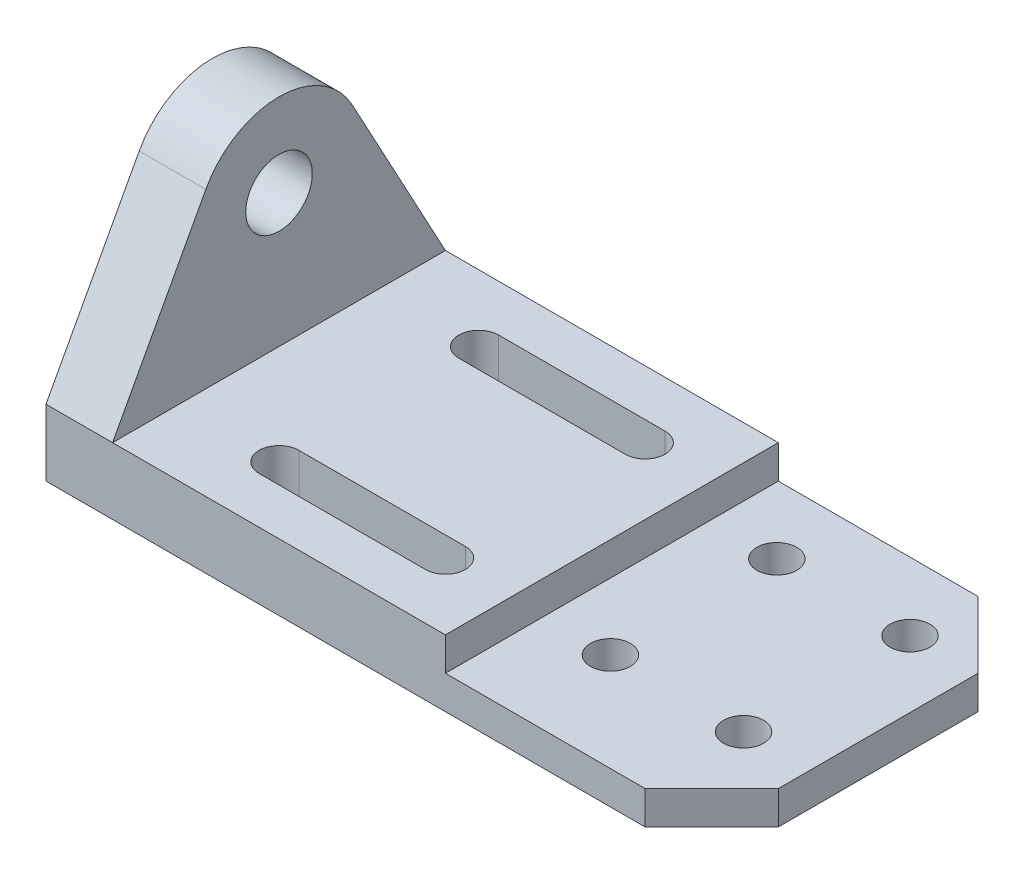
ISO-10303-21;
HEADER;
FILE_DESCRIPTION(('STEP AP214'),'2;1');
FILE_NAME('part.step','',(''),(''),'','','');
FILE_SCHEMA(('AUTOMOTIVE_DESIGN { 1 0 10303 214 1 1 1 1 }'));
ENDSEC;
DATA;
#1=APPLICATION_CONTEXT('core data for automotive mechanical design processes');
#2=APPLICATION_PROTOCOL_DEFINITION('international standard','automotive_design',2000,#1);
#3=PRODUCT_CONTEXT('',#1,'mechanical');
#4=PRODUCT('Part','Part','',(#3));
#5=PRODUCT_RELATED_PRODUCT_CATEGORY('part','',(#4));
#6=PRODUCT_DEFINITION_FORMATION('','',#4);
#7=PRODUCT_DEFINITION_CONTEXT('part definition',#1,'design');
#8=PRODUCT_DEFINITION('design','',#6,#7);
#9=PRODUCT_DEFINITION_SHAPE('','',#8);
#10=(LENGTH_UNIT() NAMED_UNIT(*) SI_UNIT(.MILLI.,.METRE.));
#11=(NAMED_UNIT(*) PLANE_ANGLE_UNIT() SI_UNIT($,.RADIAN.));
#12=(NAMED_UNIT(*) SI_UNIT($,.STERADIAN.) SOLID_ANGLE_UNIT());
#13=UNCERTAINTY_MEASURE_WITH_UNIT(LENGTH_MEASURE(1.E-05),#10,'distance_accuracy_value','');
#14=(GEOMETRIC_REPRESENTATION_CONTEXT(3) GLOBAL_UNCERTAINTY_ASSIGNED_CONTEXT((#13)) GLOBAL_UNIT_ASSIGNED_CONTEXT((#10,
#11,#12)) REPRESENTATION_CONTEXT('',''));
#15=CARTESIAN_POINT('',(0.,0.,0.));
#16=DIRECTION('',(0.,0.,1.));
#17=DIRECTION('',(1.,0.,0.));
#18=AXIS2_PLACEMENT_3D('',#15,#16,#17);
#19=CARTESIAN_POINT('',(0.,20.,0.));
#20=DIRECTION('',(0.,1.,0.));
#21=DIRECTION('',(0.,0.,1.));
#22=AXIS2_PLACEMENT_3D('',#19,#20,#21);
#23=PLANE('',#22);
#24=CARTESIAN_POINT('',(-50.,20.,30.));
#25=DIRECTION('',(0.,1.,0.));
#26=DIRECTION('',(0.,0.,1.));
#27=AXIS2_PLACEMENT_3D('',#24,#25,#26);
#28=CIRCLE('',#27,6.);
#29=CARTESIAN_POINT('',(-50.,20.,24.));
#30=VERTEX_POINT('',#29);
#31=CARTESIAN_POINT('',(-50.,20.,36.));
#32=VERTEX_POINT('',#31);
#33=EDGE_CURVE('E221',#30,#32,#28,.T.);
#34=ORIENTED_EDGE('',*,*,#33,.F.);
#35=DIRECTION('',(-1.,0.,0.));
#36=VECTOR('',#35,1.);
#37=CARTESIAN_POINT('',(-50.,20.,24.));
#38=LINE('',#37,#36);
#39=CARTESIAN_POINT('',(0.,20.,24.));
#40=VERTEX_POINT('',#39);
#41=EDGE_CURVE('E216',#40,#30,#38,.T.);
#42=ORIENTED_EDGE('',*,*,#41,.F.);
#43=CARTESIAN_POINT('',(0.,20.,30.));
#44=DIRECTION('',(0.,1.,0.));
#45=DIRECTION('',(0.,0.,1.));
#46=AXIS2_PLACEMENT_3D('',#43,#44,#45);
#47=CIRCLE('',#46,6.);
#48=CARTESIAN_POINT('',(0.,20.,36.));
#49=VERTEX_POINT('',#48);
#50=EDGE_CURVE('E227',#49,#40,#47,.T.);
#51=ORIENTED_EDGE('',*,*,#50,.F.);
#52=DIRECTION('',(1.,0.,0.));
#53=VECTOR('',#52,1.);
#54=CARTESIAN_POINT('',(-50.,20.,36.));
#55=LINE('',#54,#53);
#56=EDGE_CURVE('E228',#32,#49,#55,.T.);
#57=ORIENTED_EDGE('',*,*,#56,.F.);
#58=EDGE_LOOP('',(#34,#42,#51,#57));
#59=FACE_BOUND('',#58,.T.);
#60=CARTESIAN_POINT('',(-50.,20.,-30.));
#61=DIRECTION('',(0.,1.,0.));
#62=DIRECTION('',(0.,0.,-1.));
#63=AXIS2_PLACEMENT_3D('',#60,#61,#62);
#64=CIRCLE('',#63,6.);
#65=CARTESIAN_POINT('',(-50.,20.,-36.));
#66=VERTEX_POINT('',#65);
#67=CARTESIAN_POINT('',(-50.,20.,-24.));
#68=VERTEX_POINT('',#67);
#69=EDGE_CURVE('E209',#66,#68,#64,.T.);
#70=ORIENTED_EDGE('',*,*,#69,.F.);
#71=DIRECTION('',(-1.,0.,0.));
#72=VECTOR('',#71,1.);
#73=CARTESIAN_POINT('',(-50.,20.,-36.));
#74=LINE('',#73,#72);
#75=CARTESIAN_POINT('',(0.,20.,-36.));
#76=VERTEX_POINT('',#75);
#77=EDGE_CURVE('E250',#76,#66,#74,.T.);
#78=ORIENTED_EDGE('',*,*,#77,.F.);
#79=CARTESIAN_POINT('',(0.,20.,-30.));
#80=DIRECTION('',(0.,1.,0.));
#81=DIRECTION('',(0.,0.,-1.));
#82=AXIS2_PLACEMENT_3D('',#79,#80,#81);
#83=CIRCLE('',#82,6.);
#84=CARTESIAN_POINT('',(0.,20.,-24.));
#85=VERTEX_POINT('',#84);
#86=EDGE_CURVE('E265',#85,#76,#83,.T.);
#87=ORIENTED_EDGE('',*,*,#86,.F.);
#88=DIRECTION('',(1.,0.,0.));
#89=VECTOR('',#88,1.);
#90=CARTESIAN_POINT('',(-50.,20.,-24.));
#91=LINE('',#90,#89);
#92=EDGE_CURVE('E259',#68,#85,#91,.T.);
#93=ORIENTED_EDGE('',*,*,#92,.F.);
#94=EDGE_LOOP('',(#70,#78,#87,#93));
#95=FACE_BOUND('',#94,.T.);
#96=DIRECTION('',(-1.,0.,0.));
#97=VECTOR('',#96,1.);
#98=CARTESIAN_POINT('',(-100.,20.,-50.));
#99=LINE('',#98,#97);
#100=CARTESIAN_POINT('',(20.,20.,-50.));
#101=VERTEX_POINT('',#100);
#102=CARTESIAN_POINT('',(-80.,20.,-50.));
#103=VERTEX_POINT('',#102);
#104=EDGE_CURVE('E276',#101,#103,#99,.T.);
#105=ORIENTED_EDGE('',*,*,#104,.T.);
#106=DIRECTION('',(0.,0.,1.));
#107=VECTOR('',#106,1.);
#108=CARTESIAN_POINT('',(-80.,20.,-50.));
#109=LINE('',#108,#107);
#110=CARTESIAN_POINT('',(-80.,20.,50.));
#111=VERTEX_POINT('',#110);
#112=EDGE_CURVE('E192',#103,#111,#109,.T.);
#113=ORIENTED_EDGE('',*,*,#112,.T.);
#114=DIRECTION('',(1.,0.,0.));
#115=VECTOR('',#114,1.);
#116=CARTESIAN_POINT('',(-100.,20.,50.));
#117=LINE('',#116,#115);
#118=CARTESIAN_POINT('',(20.,20.,50.));
#119=VERTEX_POINT('',#118);
#120=EDGE_CURVE('E280',#111,#119,#117,.T.);
#121=ORIENTED_EDGE('',*,*,#120,.T.);
#122=DIRECTION('',(0.,0.,-1.));
#123=VECTOR('',#122,1.);
#124=CARTESIAN_POINT('',(20.,20.,-50.));
#125=LINE('',#124,#123);
#126=EDGE_CURVE('E277',#119,#101,#125,.T.);
#127=ORIENTED_EDGE('',*,*,#126,.T.);
#128=EDGE_LOOP('',(#105,#113,#121,#127));
#129=FACE_BOUND('',#128,.T.);
#130=ADVANCED_FACE('F41',(#59,#95,#129),#23,.T.);
#131=CARTESIAN_POINT('',(0.,10.,0.));
#132=DIRECTION('',(0.,-1.,0.));
#133=DIRECTION('',(0.,0.,-1.));
#134=AXIS2_PLACEMENT_3D('',#131,#132,#133);
#135=PLANE('',#134);
#136=CARTESIAN_POINT('',(40.,10.,20.4344291073049));
#137=DIRECTION('',(0.,1.,0.));
#138=DIRECTION('',(0.,0.,-1.));
#139=AXIS2_PLACEMENT_3D('',#136,#137,#138);
#140=CIRCLE('',#139,5.99999999999999);
#141=CARTESIAN_POINT('',(40.,10.,14.4344291073049));
#142=VERTEX_POINT('',#141);
#143=EDGE_CURVE('E355',#142,#142,#140,.T.);
#144=ORIENTED_EDGE('',*,*,#143,.F.);
#145=EDGE_LOOP('',(#144));
#146=FACE_BOUND('',#145,.T.);
#147=CARTESIAN_POINT('',(80.,10.,20.4344291073049));
#148=DIRECTION('',(0.,1.,0.));
#149=DIRECTION('',(0.,0.,-1.));
#150=AXIS2_PLACEMENT_3D('',#147,#148,#149);
#151=CIRCLE('',#150,5.99999999999998);
#152=CARTESIAN_POINT('',(80.,10.,14.4344291073049));
#153=VERTEX_POINT('',#152);
#154=EDGE_CURVE('E352',#153,#153,#151,.T.);
#155=ORIENTED_EDGE('',*,*,#154,.F.);
#156=EDGE_LOOP('',(#155));
#157=FACE_BOUND('',#156,.T.);
#158=CARTESIAN_POINT('',(80.,10.,-29.5655708926951));
#159=DIRECTION('',(0.,1.,0.));
#160=DIRECTION('',(0.,0.,1.));
#161=AXIS2_PLACEMENT_3D('',#158,#159,#160);
#162=CIRCLE('',#161,6.);
#163=CARTESIAN_POINT('',(80.,10.,-23.5655708926951));
#164=VERTEX_POINT('',#163);
#165=EDGE_CURVE('E353',#164,#164,#162,.T.);
#166=ORIENTED_EDGE('',*,*,#165,.F.);
#167=EDGE_LOOP('',(#166));
#168=FACE_BOUND('',#167,.T.);
#169=CARTESIAN_POINT('',(40.,10.,-29.5655708926951));
#170=DIRECTION('',(0.,1.,0.));
#171=DIRECTION('',(0.,0.,1.));
#172=AXIS2_PLACEMENT_3D('',#169,#170,#171);
#173=CIRCLE('',#172,6.);
#174=CARTESIAN_POINT('',(40.,10.,-23.5655708926951));
#175=VERTEX_POINT('',#174);
#176=EDGE_CURVE('E334',#175,#175,#173,.T.);
#177=ORIENTED_EDGE('',*,*,#176,.F.);
#178=EDGE_LOOP('',(#177));
#179=FACE_BOUND('',#178,.T.);
#180=DIRECTION('',(0.,0.,-1.));
#181=VECTOR('',#180,1.);
#182=CARTESIAN_POINT('',(100.,10.,50.));
#183=LINE('',#182,#181);
#184=CARTESIAN_POINT('',(100.,10.,30.));
#185=VERTEX_POINT('',#184);
#186=CARTESIAN_POINT('',(100.,10.,-29.9999999999999));
#187=VERTEX_POINT('',#186);
#188=EDGE_CURVE('E292',#185,#187,#183,.T.);
#189=ORIENTED_EDGE('',*,*,#188,.T.);
#190=DIRECTION('',(0.707106781186547,0.,0.707106781186549));
#191=VECTOR('',#190,1.);
#192=CARTESIAN_POINT('',(80.,10.,-50.));
#193=LINE('',#192,#191);
#194=CARTESIAN_POINT('',(80.,10.,-50.));
#195=VERTEX_POINT('',#194);
#196=EDGE_CURVE('E11',#187,#195,#193,.F.);
#197=ORIENTED_EDGE('',*,*,#196,.T.);
#198=DIRECTION('',(-1.,0.,0.));
#199=VECTOR('',#198,1.);
#200=CARTESIAN_POINT('',(-100.,10.,-50.));
#201=LINE('',#200,#199);
#202=CARTESIAN_POINT('',(20.,10.,-50.));
#203=VERTEX_POINT('',#202);
#204=EDGE_CURVE('E294',#195,#203,#201,.T.);
#205=ORIENTED_EDGE('',*,*,#204,.T.);
#206=DIRECTION('',(0.,0.,-1.));
#207=VECTOR('',#206,1.);
#208=CARTESIAN_POINT('',(20.,10.,-50.));
#209=LINE('',#208,#207);
#210=CARTESIAN_POINT('',(20.,10.,50.));
#211=VERTEX_POINT('',#210);
#212=EDGE_CURVE('E240',#211,#203,#209,.T.);
#213=ORIENTED_EDGE('',*,*,#212,.F.);
#214=DIRECTION('',(1.,0.,0.));
#215=VECTOR('',#214,1.);
#216=CARTESIAN_POINT('',(-100.,10.,50.));
#217=LINE('',#216,#215);
#218=CARTESIAN_POINT('',(79.9999999999999,10.,50.));
#219=VERTEX_POINT('',#218);
#220=EDGE_CURVE('E300',#211,#219,#217,.T.);
#221=ORIENTED_EDGE('',*,*,#220,.T.);
#222=DIRECTION('',(-0.707106781186549,0.,0.707106781186547));
#223=VECTOR('',#222,1.);
#224=CARTESIAN_POINT('',(100.,10.,30.));
#225=LINE('',#224,#223);
#226=EDGE_CURVE('E321',#219,#185,#225,.F.);
#227=ORIENTED_EDGE('',*,*,#226,.T.);
#228=EDGE_LOOP('',(#189,#197,#205,#213,#221,#227));
#229=FACE_BOUND('',#228,.T.);
#230=ADVANCED_FACE('F361',(#146,#157,#168,#179,#229),#135,.F.);
#231=CARTESIAN_POINT('',(100.,10.,50.));
#232=DIRECTION('',(-1.,0.,0.));
#233=DIRECTION('',(0.,0.,1.));
#234=AXIS2_PLACEMENT_3D('',#231,#232,#233);
#235=PLANE('',#234);
#236=DIRECTION('',(0.,0.,-1.));
#237=VECTOR('',#236,1.);
#238=CARTESIAN_POINT('',(100.,0.,50.));
#239=LINE('',#238,#237);
#240=CARTESIAN_POINT('',(100.,0.,30.));
#241=VERTEX_POINT('',#240);
#242=CARTESIAN_POINT('',(100.,0.,-29.9999999999999));
#243=VERTEX_POINT('',#242);
#244=EDGE_CURVE('E288',#241,#243,#239,.T.);
#245=ORIENTED_EDGE('',*,*,#244,.T.);
#246=DIRECTION('',(0.,1.,0.));
#247=VECTOR('',#246,1.);
#248=CARTESIAN_POINT('',(100.,10.,-29.9999999999999));
#249=LINE('',#248,#247);
#250=EDGE_CURVE('E51',#243,#187,#249,.T.);
#251=ORIENTED_EDGE('',*,*,#250,.T.);
#252=ORIENTED_EDGE('',*,*,#188,.F.);
#253=DIRECTION('',(0.,-1.,0.));
#254=VECTOR('',#253,1.);
#255=CARTESIAN_POINT('',(100.,10.,30.));
#256=LINE('',#255,#254);
#257=EDGE_CURVE('E314',#185,#241,#256,.T.);
#258=ORIENTED_EDGE('',*,*,#257,.T.);
#259=EDGE_LOOP('',(#245,#251,#252,#258));
#260=FACE_BOUND('',#259,.T.);
#261=ADVANCED_FACE('F368',(#260),#235,.F.);
#262=CARTESIAN_POINT('',(-100.,10.,-50.));
#263=DIRECTION('',(0.,0.,1.));
#264=DIRECTION('',(1.,0.,0.));
#265=AXIS2_PLACEMENT_3D('',#262,#263,#264);
#266=PLANE('',#265);
#267=ORIENTED_EDGE('',*,*,#204,.F.);
#268=DIRECTION('',(0.,-1.,0.));
#269=VECTOR('',#268,1.);
#270=CARTESIAN_POINT('',(80.,10.,-50.));
#271=LINE('',#270,#269);
#272=CARTESIAN_POINT('',(80.,0.,-50.));
#273=VERTEX_POINT('',#272);
#274=EDGE_CURVE('E323',#195,#273,#271,.T.);
#275=ORIENTED_EDGE('',*,*,#274,.T.);
#276=DIRECTION('',(-1.,0.,0.));
#277=VECTOR('',#276,1.);
#278=CARTESIAN_POINT('',(-100.,0.,-50.));
#279=LINE('',#278,#277);
#280=CARTESIAN_POINT('',(-100.,0.,-50.));
#281=VERTEX_POINT('',#280);
#282=EDGE_CURVE('E305',#273,#281,#279,.T.);
#283=ORIENTED_EDGE('',*,*,#282,.T.);
#284=DIRECTION('',(0.,-1.,0.));
#285=VECTOR('',#284,1.);
#286=CARTESIAN_POINT('',(-100.,10.,-50.));
#287=LINE('',#286,#285);
#288=CARTESIAN_POINT('',(-100.,20.,-50.));
#289=VERTEX_POINT('',#288);
#290=EDGE_CURVE('E313',#289,#281,#287,.T.);
#291=ORIENTED_EDGE('',*,*,#290,.F.);
#292=DIRECTION('',(-1.,0.,0.));
#293=VECTOR('',#292,1.);
#294=CARTESIAN_POINT('',(-80.,20.,-50.));
#295=LINE('',#294,#293);
#296=EDGE_CURVE('E188',#103,#289,#295,.T.);
#297=ORIENTED_EDGE('',*,*,#296,.F.);
#298=ORIENTED_EDGE('',*,*,#104,.F.);
#299=DIRECTION('',(0.,-1.,0.));
#300=VECTOR('',#299,1.);
#301=CARTESIAN_POINT('',(20.,20.,-50.));
#302=LINE('',#301,#300);
#303=EDGE_CURVE('E285',#101,#203,#302,.T.);
#304=ORIENTED_EDGE('',*,*,#303,.T.);
#305=EDGE_LOOP('',(#267,#275,#283,#291,#297,#298,#304));
#306=FACE_BOUND('',#305,.T.);
#307=ADVANCED_FACE('F385',(#306),#266,.F.);
#308=CARTESIAN_POINT('',(-100.,10.,50.));
#309=DIRECTION('',(1.,0.,0.));
#310=DIRECTION('',(0.,0.,-1.));
#311=AXIS2_PLACEMENT_3D('',#308,#309,#310);
#312=PLANE('',#311);
#313=DIRECTION('',(0.,0.,1.));
#314=VECTOR('',#313,1.);
#315=CARTESIAN_POINT('',(-100.,0.,50.));
#316=LINE('',#315,#314);
#317=CARTESIAN_POINT('',(-100.,0.,50.));
#318=VERTEX_POINT('',#317);
#319=EDGE_CURVE('E303',#281,#318,#316,.T.);
#320=ORIENTED_EDGE('',*,*,#319,.T.);
#321=DIRECTION('',(0.,-1.,0.));
#322=VECTOR('',#321,1.);
#323=CARTESIAN_POINT('',(-100.,10.,50.));
#324=LINE('',#323,#322);
#325=CARTESIAN_POINT('',(-100.,20.,50.));
#326=VERTEX_POINT('',#325);
#327=EDGE_CURVE('E297',#326,#318,#324,.T.);
#328=ORIENTED_EDGE('',*,*,#327,.F.);
#329=DIRECTION('',(0.,0.879991518173248,-0.474989397716561));
#330=VECTOR('',#329,1.);
#331=CARTESIAN_POINT('',(-100.,71.874734942914,21.9997879543312));
#332=LINE('',#331,#330);
#333=CARTESIAN_POINT('',(-100.,71.874734942914,21.9997879543312));
#334=VERTEX_POINT('',#333);
#335=EDGE_CURVE('E193',#326,#334,#332,.T.);
#336=ORIENTED_EDGE('',*,*,#335,.T.);
#337=CARTESIAN_POINT('',(-100.,60.,0.));
#338=DIRECTION('',(-1.,0.,0.));
#339=DIRECTION('',(0.,0.,1.));
#340=AXIS2_PLACEMENT_3D('',#337,#338,#339);
#341=CIRCLE('',#340,25.);
#342=CARTESIAN_POINT('',(-100.,71.874734942914,-21.9997879543312));
#343=VERTEX_POINT('',#342);
#344=EDGE_CURVE('E202',#334,#343,#341,.T.);
#345=ORIENTED_EDGE('',*,*,#344,.T.);
#346=DIRECTION('',(0.,-0.879991518173249,-0.47498939771656));
#347=VECTOR('',#346,1.);
#348=CARTESIAN_POINT('',(-100.,71.874734942914,-21.9997879543312));
#349=LINE('',#348,#347);
#350=EDGE_CURVE('E182',#343,#289,#349,.T.);
#351=ORIENTED_EDGE('',*,*,#350,.T.);
#352=ORIENTED_EDGE('',*,*,#290,.T.);
#353=EDGE_LOOP('',(#320,#328,#336,#345,#351,#352));
#354=FACE_BOUND('',#353,.T.);
#355=CARTESIAN_POINT('',(-100.,60.,0.));
#356=DIRECTION('',(-1.,0.,0.));
#357=DIRECTION('',(0.,0.,1.));
#358=AXIS2_PLACEMENT_3D('',#355,#356,#357);
#359=CIRCLE('',#358,10.);
#360=CARTESIAN_POINT('',(-100.,60.,10.));
#361=VERTEX_POINT('',#360);
#362=EDGE_CURVE('E199',#361,#361,#359,.T.);
#363=ORIENTED_EDGE('',*,*,#362,.F.);
#364=EDGE_LOOP('',(#363));
#365=FACE_BOUND('',#364,.T.);
#366=ADVANCED_FACE('F393',(#354,#365),#312,.F.);
#367=CARTESIAN_POINT('',(-100.,10.,50.));
#368=DIRECTION('',(0.,0.,-1.));
#369=DIRECTION('',(-1.,0.,0.));
#370=AXIS2_PLACEMENT_3D('',#367,#368,#369);
#371=PLANE('',#370);
#372=DIRECTION('',(1.,0.,0.));
#373=VECTOR('',#372,1.);
#374=CARTESIAN_POINT('',(-100.,0.,50.));
#375=LINE('',#374,#373);
#376=CARTESIAN_POINT('',(79.9999999999999,0.,50.));
#377=VERTEX_POINT('',#376);
#378=EDGE_CURVE('E293',#318,#377,#375,.T.);
#379=ORIENTED_EDGE('',*,*,#378,.T.);
#380=DIRECTION('',(0.,1.,0.));
#381=VECTOR('',#380,1.);
#382=CARTESIAN_POINT('',(79.9999999999999,10.,50.));
#383=LINE('',#382,#381);
#384=EDGE_CURVE('E317',#377,#219,#383,.T.);
#385=ORIENTED_EDGE('',*,*,#384,.T.);
#386=ORIENTED_EDGE('',*,*,#220,.F.);
#387=DIRECTION('',(0.,-1.,0.));
#388=VECTOR('',#387,1.);
#389=CARTESIAN_POINT('',(20.,20.,50.));
#390=LINE('',#389,#388);
#391=EDGE_CURVE('E289',#119,#211,#390,.T.);
#392=ORIENTED_EDGE('',*,*,#391,.F.);
#393=ORIENTED_EDGE('',*,*,#120,.F.);
#394=EDGE_CURVE('E273',#326,#111,#117,.T.);
#395=ORIENTED_EDGE('',*,*,#394,.F.);
#396=ORIENTED_EDGE('',*,*,#327,.T.);
#397=EDGE_LOOP('',(#379,#385,#386,#392,#393,#395,#396));
#398=FACE_BOUND('',#397,.T.);
#399=ADVANCED_FACE('F392',(#398),#371,.F.);
#400=CARTESIAN_POINT('',(0.,0.,0.));
#401=DIRECTION('',(0.,-1.,0.));
#402=DIRECTION('',(0.,0.,-1.));
#403=AXIS2_PLACEMENT_3D('',#400,#401,#402);
#404=PLANE('',#403);
#405=CARTESIAN_POINT('',(40.,0.,20.4344291073049));
#406=DIRECTION('',(0.,-1.,0.));
#407=DIRECTION('',(0.,0.,-1.));
#408=AXIS2_PLACEMENT_3D('',#405,#406,#407);
#409=CIRCLE('',#408,5.99999999999999);
#410=CARTESIAN_POINT('',(40.,0.,14.4344291073049));
#411=VERTEX_POINT('',#410);
#412=EDGE_CURVE('E46',#411,#411,#409,.T.);
#413=ORIENTED_EDGE('',*,*,#412,.F.);
#414=EDGE_LOOP('',(#413));
#415=FACE_BOUND('',#414,.T.);
#416=CARTESIAN_POINT('',(80.,0.,20.4344291073049));
#417=DIRECTION('',(0.,-1.,0.));
#418=DIRECTION('',(0.,0.,-1.));
#419=AXIS2_PLACEMENT_3D('',#416,#417,#418);
#420=CIRCLE('',#419,5.99999999999998);
#421=CARTESIAN_POINT('',(80.,0.,14.4344291073049));
#422=VERTEX_POINT('',#421);
#423=EDGE_CURVE('E333',#422,#422,#420,.T.);
#424=ORIENTED_EDGE('',*,*,#423,.F.);
#425=EDGE_LOOP('',(#424));
#426=FACE_BOUND('',#425,.T.);
#427=CARTESIAN_POINT('',(80.,0.,-29.5655708926951));
#428=DIRECTION('',(0.,-1.,0.));
#429=DIRECTION('',(0.,0.,-1.));
#430=AXIS2_PLACEMENT_3D('',#427,#428,#429);
#431=CIRCLE('',#430,6.);
#432=CARTESIAN_POINT('',(80.,0.,-35.5655708926951));
#433=VERTEX_POINT('',#432);
#434=EDGE_CURVE('E335',#433,#433,#431,.T.);
#435=ORIENTED_EDGE('',*,*,#434,.F.);
#436=EDGE_LOOP('',(#435));
#437=FACE_BOUND('',#436,.T.);
#438=CARTESIAN_POINT('',(40.,0.,-29.5655708926951));
#439=DIRECTION('',(0.,-1.,0.));
#440=DIRECTION('',(0.,0.,-1.));
#441=AXIS2_PLACEMENT_3D('',#438,#439,#440);
#442=CIRCLE('',#441,6.);
#443=CARTESIAN_POINT('',(40.,0.,-35.5655708926951));
#444=VERTEX_POINT('',#443);
#445=EDGE_CURVE('E328',#444,#444,#442,.T.);
#446=ORIENTED_EDGE('',*,*,#445,.F.);
#447=EDGE_LOOP('',(#446));
#448=FACE_BOUND('',#447,.T.);
#449=CARTESIAN_POINT('',(-50.,0.,30.));
#450=DIRECTION('',(0.,1.,0.));
#451=DIRECTION('',(0.,0.,1.));
#452=AXIS2_PLACEMENT_3D('',#449,#450,#451);
#453=CIRCLE('',#452,6.);
#454=CARTESIAN_POINT('',(-50.,0.,24.));
#455=VERTEX_POINT('',#454);
#456=CARTESIAN_POINT('',(-50.,0.,36.));
#457=VERTEX_POINT('',#456);
#458=EDGE_CURVE('E215',#455,#457,#453,.T.);
#459=ORIENTED_EDGE('',*,*,#458,.T.);
#460=DIRECTION('',(1.,0.,0.));
#461=VECTOR('',#460,1.);
#462=CARTESIAN_POINT('',(-50.,0.,36.));
#463=LINE('',#462,#461);
#464=CARTESIAN_POINT('',(0.,0.,36.));
#465=VERTEX_POINT('',#464);
#466=EDGE_CURVE('E214',#457,#465,#463,.T.);
#467=ORIENTED_EDGE('',*,*,#466,.T.);
#468=CARTESIAN_POINT('',(0.,0.,30.));
#469=DIRECTION('',(0.,1.,0.));
#470=DIRECTION('',(0.,0.,1.));
#471=AXIS2_PLACEMENT_3D('',#468,#469,#470);
#472=CIRCLE('',#471,6.);
#473=CARTESIAN_POINT('',(0.,0.,24.));
#474=VERTEX_POINT('',#473);
#475=EDGE_CURVE('E69',#465,#474,#472,.T.);
#476=ORIENTED_EDGE('',*,*,#475,.T.);
#477=DIRECTION('',(-1.,0.,0.));
#478=VECTOR('',#477,1.);
#479=CARTESIAN_POINT('',(-50.,0.,24.));
#480=LINE('',#479,#478);
#481=EDGE_CURVE('E219',#474,#455,#480,.T.);
#482=ORIENTED_EDGE('',*,*,#481,.T.);
#483=EDGE_LOOP('',(#459,#467,#476,#482));
#484=FACE_BOUND('',#483,.T.);
#485=CARTESIAN_POINT('',(-50.,0.,-30.));
#486=DIRECTION('',(0.,1.,0.));
#487=DIRECTION('',(0.,0.,-1.));
#488=AXIS2_PLACEMENT_3D('',#485,#486,#487);
#489=CIRCLE('',#488,6.);
#490=CARTESIAN_POINT('',(-50.,0.,-36.));
#491=VERTEX_POINT('',#490);
#492=CARTESIAN_POINT('',(-50.,0.,-24.));
#493=VERTEX_POINT('',#492);
#494=EDGE_CURVE('E244',#491,#493,#489,.T.);
#495=ORIENTED_EDGE('',*,*,#494,.T.);
#496=DIRECTION('',(1.,0.,0.));
#497=VECTOR('',#496,1.);
#498=CARTESIAN_POINT('',(-50.,0.,-24.));
#499=LINE('',#498,#497);
#500=CARTESIAN_POINT('',(0.,0.,-24.));
#501=VERTEX_POINT('',#500);
#502=EDGE_CURVE('E249',#493,#501,#499,.T.);
#503=ORIENTED_EDGE('',*,*,#502,.T.);
#504=CARTESIAN_POINT('',(0.,0.,-30.));
#505=DIRECTION('',(0.,1.,0.));
#506=DIRECTION('',(0.,0.,-1.));
#507=AXIS2_PLACEMENT_3D('',#504,#505,#506);
#508=CIRCLE('',#507,6.);
#509=CARTESIAN_POINT('',(0.,0.,-36.));
#510=VERTEX_POINT('',#509);
#511=EDGE_CURVE('E253',#501,#510,#508,.T.);
#512=ORIENTED_EDGE('',*,*,#511,.T.);
#513=DIRECTION('',(-1.,0.,0.));
#514=VECTOR('',#513,1.);
#515=CARTESIAN_POINT('',(-50.,0.,-36.));
#516=LINE('',#515,#514);
#517=EDGE_CURVE('E255',#510,#491,#516,.T.);
#518=ORIENTED_EDGE('',*,*,#517,.T.);
#519=EDGE_LOOP('',(#495,#503,#512,#518));
#520=FACE_BOUND('',#519,.T.);
#521=ORIENTED_EDGE('',*,*,#282,.F.);
#522=DIRECTION('',(-0.707106781186547,0.,-0.707106781186549));
#523=VECTOR('',#522,1.);
#524=CARTESIAN_POINT('',(65.0000000000001,0.,-64.9999999999999));
#525=LINE('',#524,#523);
#526=EDGE_CURVE('E326',#273,#243,#525,.F.);
#527=ORIENTED_EDGE('',*,*,#526,.T.);
#528=ORIENTED_EDGE('',*,*,#244,.F.);
#529=DIRECTION('',(0.707106781186549,0.,-0.707106781186547));
#530=VECTOR('',#529,1.);
#531=CARTESIAN_POINT('',(64.9999999999999,0.,65.0000000000001));
#532=LINE('',#531,#530);
#533=EDGE_CURVE('E320',#241,#377,#532,.F.);
#534=ORIENTED_EDGE('',*,*,#533,.T.);
#535=ORIENTED_EDGE('',*,*,#378,.F.);
#536=ORIENTED_EDGE('',*,*,#319,.F.);
#537=EDGE_LOOP('',(#521,#527,#528,#534,#535,#536));
#538=FACE_BOUND('',#537,.T.);
#539=ADVANCED_FACE('F387',(#415,#426,#437,#448,#484,#520,#538),#404,.T.);
#540=CARTESIAN_POINT('',(20.,20.,-50.));
#541=DIRECTION('',(-1.,0.,0.));
#542=DIRECTION('',(0.,0.,1.));
#543=AXIS2_PLACEMENT_3D('',#540,#541,#542);
#544=PLANE('',#543);
#545=ORIENTED_EDGE('',*,*,#212,.T.);
#546=ORIENTED_EDGE('',*,*,#303,.F.);
#547=ORIENTED_EDGE('',*,*,#126,.F.);
#548=ORIENTED_EDGE('',*,*,#391,.T.);
#549=EDGE_LOOP('',(#545,#546,#547,#548));
#550=FACE_BOUND('',#549,.T.);
#551=ADVANCED_FACE('F408',(#550),#544,.F.);
#552=CARTESIAN_POINT('',(100.,10.,30.));
#553=DIRECTION('',(-0.707106781186547,0.,-0.707106781186549));
#554=DIRECTION('',(0.,-1.,0.));
#555=AXIS2_PLACEMENT_3D('',#552,#553,#554);
#556=PLANE('',#555);
#557=ORIENTED_EDGE('',*,*,#226,.F.);
#558=ORIENTED_EDGE('',*,*,#384,.F.);
#559=ORIENTED_EDGE('',*,*,#533,.F.);
#560=ORIENTED_EDGE('',*,*,#257,.F.);
#561=EDGE_LOOP('',(#557,#558,#559,#560));
#562=FACE_BOUND('',#561,.T.);
#563=ADVANCED_FACE('F409',(#562),#556,.F.);
#564=CARTESIAN_POINT('',(80.,10.,-50.));
#565=DIRECTION('',(-0.707106781186549,0.,0.707106781186547));
#566=DIRECTION('',(0.,-1.,0.));
#567=AXIS2_PLACEMENT_3D('',#564,#565,#566);
#568=PLANE('',#567);
#569=ORIENTED_EDGE('',*,*,#196,.F.);
#570=ORIENTED_EDGE('',*,*,#250,.F.);
#571=ORIENTED_EDGE('',*,*,#526,.F.);
#572=ORIENTED_EDGE('',*,*,#274,.F.);
#573=EDGE_LOOP('',(#569,#570,#571,#572));
#574=FACE_BOUND('',#573,.T.);
#575=ADVANCED_FACE('F42',(#574),#568,.F.);
#576=CARTESIAN_POINT('',(-50.,0.,-30.));
#577=DIRECTION('',(0.,1.,0.));
#578=DIRECTION('',(0.,0.,1.));
#579=AXIS2_PLACEMENT_3D('',#576,#577,#578);
#580=CYLINDRICAL_SURFACE('',#579,6.);
#581=ORIENTED_EDGE('',*,*,#69,.T.);
#582=DIRECTION('',(0.,1.,0.));
#583=VECTOR('',#582,1.);
#584=CARTESIAN_POINT('',(-50.,0.,-24.));
#585=LINE('',#584,#583);
#586=EDGE_CURVE('E260',#493,#68,#585,.T.);
#587=ORIENTED_EDGE('',*,*,#586,.F.);
#588=ORIENTED_EDGE('',*,*,#494,.F.);
#589=DIRECTION('',(0.,1.,0.));
#590=VECTOR('',#589,1.);
#591=CARTESIAN_POINT('',(-50.,0.,-36.));
#592=LINE('',#591,#590);
#593=EDGE_CURVE('E230',#491,#66,#592,.T.);
#594=ORIENTED_EDGE('',*,*,#593,.T.);
#595=EDGE_LOOP('',(#581,#587,#588,#594));
#596=FACE_BOUND('',#595,.T.);
#597=ADVANCED_FACE('F428',(#596),#580,.F.);
#598=CARTESIAN_POINT('',(-50.,0.,-36.));
#599=DIRECTION('',(0.,0.,-1.));
#600=DIRECTION('',(-1.,0.,0.));
#601=AXIS2_PLACEMENT_3D('',#598,#599,#600);
#602=PLANE('',#601);
#603=ORIENTED_EDGE('',*,*,#77,.T.);
#604=ORIENTED_EDGE('',*,*,#593,.F.);
#605=ORIENTED_EDGE('',*,*,#517,.F.);
#606=DIRECTION('',(0.,1.,0.));
#607=VECTOR('',#606,1.);
#608=CARTESIAN_POINT('',(0.,0.,-36.));
#609=LINE('',#608,#607);
#610=EDGE_CURVE('E268',#510,#76,#609,.T.);
#611=ORIENTED_EDGE('',*,*,#610,.T.);
#612=EDGE_LOOP('',(#603,#604,#605,#611));
#613=FACE_BOUND('',#612,.T.);
#614=ADVANCED_FACE('F595',(#613),#602,.F.);
#615=CARTESIAN_POINT('',(0.,0.,-30.));
#616=DIRECTION('',(0.,1.,0.));
#617=DIRECTION('',(0.,0.,1.));
#618=AXIS2_PLACEMENT_3D('',#615,#616,#617);
#619=CYLINDRICAL_SURFACE('',#618,6.);
#620=ORIENTED_EDGE('',*,*,#86,.T.);
#621=ORIENTED_EDGE('',*,*,#610,.F.);
#622=ORIENTED_EDGE('',*,*,#511,.F.);
#623=DIRECTION('',(0.,1.,0.));
#624=VECTOR('',#623,1.);
#625=CARTESIAN_POINT('',(0.,0.,-24.));
#626=LINE('',#625,#624);
#627=EDGE_CURVE('E269',#501,#85,#626,.T.);
#628=ORIENTED_EDGE('',*,*,#627,.T.);
#629=EDGE_LOOP('',(#620,#621,#622,#628));
#630=FACE_BOUND('',#629,.T.);
#631=ADVANCED_FACE('F585',(#630),#619,.F.);
#632=CARTESIAN_POINT('',(-50.,0.,-24.));
#633=DIRECTION('',(0.,0.,1.));
#634=DIRECTION('',(1.,0.,0.));
#635=AXIS2_PLACEMENT_3D('',#632,#633,#634);
#636=PLANE('',#635);
#637=ORIENTED_EDGE('',*,*,#92,.T.);
#638=ORIENTED_EDGE('',*,*,#627,.F.);
#639=ORIENTED_EDGE('',*,*,#502,.F.);
#640=ORIENTED_EDGE('',*,*,#586,.T.);
#641=EDGE_LOOP('',(#637,#638,#639,#640));
#642=FACE_BOUND('',#641,.T.);
#643=ADVANCED_FACE('F572',(#642),#636,.F.);
#644=CARTESIAN_POINT('',(-50.,0.,30.));
#645=DIRECTION('',(0.,1.,0.));
#646=DIRECTION('',(0.,0.,1.));
#647=AXIS2_PLACEMENT_3D('',#644,#645,#646);
#648=CYLINDRICAL_SURFACE('',#647,6.);
#649=ORIENTED_EDGE('',*,*,#33,.T.);
#650=DIRECTION('',(0.,1.,0.));
#651=VECTOR('',#650,1.);
#652=CARTESIAN_POINT('',(-50.,0.,36.));
#653=LINE('',#652,#651);
#654=EDGE_CURVE('E224',#457,#32,#653,.T.);
#655=ORIENTED_EDGE('',*,*,#654,.F.);
#656=ORIENTED_EDGE('',*,*,#458,.F.);
#657=DIRECTION('',(0.,1.,0.));
#658=VECTOR('',#657,1.);
#659=CARTESIAN_POINT('',(-50.,0.,24.));
#660=LINE('',#659,#658);
#661=EDGE_CURVE('E233',#455,#30,#660,.T.);
#662=ORIENTED_EDGE('',*,*,#661,.T.);
#663=EDGE_LOOP('',(#649,#655,#656,#662));
#664=FACE_BOUND('',#663,.T.);
#665=ADVANCED_FACE('F567',(#664),#648,.F.);
#666=CARTESIAN_POINT('',(-50.,0.,24.));
#667=DIRECTION('',(0.,0.,-1.));
#668=DIRECTION('',(-1.,0.,0.));
#669=AXIS2_PLACEMENT_3D('',#666,#667,#668);
#670=PLANE('',#669);
#671=ORIENTED_EDGE('',*,*,#41,.T.);
#672=ORIENTED_EDGE('',*,*,#661,.F.);
#673=ORIENTED_EDGE('',*,*,#481,.F.);
#674=DIRECTION('',(0.,1.,0.));
#675=VECTOR('',#674,1.);
#676=CARTESIAN_POINT('',(0.,0.,24.));
#677=LINE('',#676,#675);
#678=EDGE_CURVE('E236',#474,#40,#677,.T.);
#679=ORIENTED_EDGE('',*,*,#678,.T.);
#680=EDGE_LOOP('',(#671,#672,#673,#679));
#681=FACE_BOUND('',#680,.T.);
#682=ADVANCED_FACE('F556',(#681),#670,.F.);
#683=CARTESIAN_POINT('',(0.,0.,30.));
#684=DIRECTION('',(0.,1.,0.));
#685=DIRECTION('',(0.,0.,1.));
#686=AXIS2_PLACEMENT_3D('',#683,#684,#685);
#687=CYLINDRICAL_SURFACE('',#686,6.);
#688=ORIENTED_EDGE('',*,*,#50,.T.);
#689=ORIENTED_EDGE('',*,*,#678,.F.);
#690=ORIENTED_EDGE('',*,*,#475,.F.);
#691=DIRECTION('',(0.,1.,0.));
#692=VECTOR('',#691,1.);
#693=CARTESIAN_POINT('',(0.,0.,36.));
#694=LINE('',#693,#692);
#695=EDGE_CURVE('E238',#465,#49,#694,.T.);
#696=ORIENTED_EDGE('',*,*,#695,.T.);
#697=EDGE_LOOP('',(#688,#689,#690,#696));
#698=FACE_BOUND('',#697,.T.);
#699=ADVANCED_FACE('F548',(#698),#687,.F.);
#700=CARTESIAN_POINT('',(-50.,0.,36.));
#701=DIRECTION('',(0.,0.,1.));
#702=DIRECTION('',(1.,0.,0.));
#703=AXIS2_PLACEMENT_3D('',#700,#701,#702);
#704=PLANE('',#703);
#705=ORIENTED_EDGE('',*,*,#56,.T.);
#706=ORIENTED_EDGE('',*,*,#695,.F.);
#707=ORIENTED_EDGE('',*,*,#466,.F.);
#708=ORIENTED_EDGE('',*,*,#654,.T.);
#709=EDGE_LOOP('',(#705,#706,#707,#708));
#710=FACE_BOUND('',#709,.T.);
#711=ADVANCED_FACE('F457',(#710),#704,.F.);
#712=CARTESIAN_POINT('',(-80.,60.,0.));
#713=DIRECTION('',(-1.,0.,0.));
#714=DIRECTION('',(0.,0.,1.));
#715=AXIS2_PLACEMENT_3D('',#712,#713,#714);
#716=CYLINDRICAL_SURFACE('',#715,25.);
#717=ORIENTED_EDGE('',*,*,#344,.F.);
#718=DIRECTION('',(-1.,0.,0.));
#719=VECTOR('',#718,1.);
#720=CARTESIAN_POINT('',(-80.,71.874734942914,21.9997879543312));
#721=LINE('',#720,#719);
#722=CARTESIAN_POINT('',(-80.,71.874734942914,21.9997879543312));
#723=VERTEX_POINT('',#722);
#724=EDGE_CURVE('E191',#723,#334,#721,.T.);
#725=ORIENTED_EDGE('',*,*,#724,.F.);
#726=CARTESIAN_POINT('',(-80.,60.,0.));
#727=DIRECTION('',(-1.,0.,0.));
#728=DIRECTION('',(0.,0.,1.));
#729=AXIS2_PLACEMENT_3D('',#726,#727,#728);
#730=CIRCLE('',#729,25.);
#731=CARTESIAN_POINT('',(-80.,71.874734942914,-21.9997879543312));
#732=VERTEX_POINT('',#731);
#733=EDGE_CURVE('E189',#723,#732,#730,.T.);
#734=ORIENTED_EDGE('',*,*,#733,.T.);
#735=DIRECTION('',(-1.,0.,0.));
#736=VECTOR('',#735,1.);
#737=CARTESIAN_POINT('',(-80.,71.874734942914,-21.9997879543312));
#738=LINE('',#737,#736);
#739=EDGE_CURVE('E172',#732,#343,#738,.T.);
#740=ORIENTED_EDGE('',*,*,#739,.T.);
#741=EDGE_LOOP('',(#717,#725,#734,#740));
#742=FACE_BOUND('',#741,.T.);
#743=ADVANCED_FACE('F195',(#742),#716,.T.);
#744=CARTESIAN_POINT('',(-80.,71.874734942914,21.9997879543312));
#745=DIRECTION('',(0.,0.474989397716561,0.879991518173248));
#746=DIRECTION('',(0.,-0.879991518173249,0.474989397716561));
#747=AXIS2_PLACEMENT_3D('',#744,#745,#746);
#748=PLANE('',#747);
#749=ORIENTED_EDGE('',*,*,#335,.F.);
#750=ORIENTED_EDGE('',*,*,#394,.T.);
#751=DIRECTION('',(0.,0.879991518173248,-0.474989397716561));
#752=VECTOR('',#751,1.);
#753=CARTESIAN_POINT('',(-80.,71.874734942914,21.9997879543312));
#754=LINE('',#753,#752);
#755=EDGE_CURVE('E56',#111,#723,#754,.T.);
#756=ORIENTED_EDGE('',*,*,#755,.T.);
#757=ORIENTED_EDGE('',*,*,#724,.T.);
#758=EDGE_LOOP('',(#749,#750,#756,#757));
#759=FACE_BOUND('',#758,.T.);
#760=ADVANCED_FACE('F398',(#759),#748,.T.);
#761=CARTESIAN_POINT('',(-80.,71.874734942914,-21.9997879543312));
#762=DIRECTION('',(0.,0.47498939771656,-0.879991518173249));
#763=DIRECTION('',(0.,0.879991518173249,0.47498939771656));
#764=AXIS2_PLACEMENT_3D('',#761,#762,#763);
#765=PLANE('',#764);
#766=ORIENTED_EDGE('',*,*,#350,.F.);
#767=ORIENTED_EDGE('',*,*,#739,.F.);
#768=DIRECTION('',(0.,-0.879991518173249,-0.47498939771656));
#769=VECTOR('',#768,1.);
#770=CARTESIAN_POINT('',(-80.,71.874734942914,-21.9997879543312));
#771=LINE('',#770,#769);
#772=EDGE_CURVE('E180',#732,#103,#771,.T.);
#773=ORIENTED_EDGE('',*,*,#772,.T.);
#774=ORIENTED_EDGE('',*,*,#296,.T.);
#775=EDGE_LOOP('',(#766,#767,#773,#774));
#776=FACE_BOUND('',#775,.T.);
#777=ADVANCED_FACE('F179',(#776),#765,.T.);
#778=CARTESIAN_POINT('',(-80.,60.,0.));
#779=DIRECTION('',(-1.,0.,0.));
#780=DIRECTION('',(0.,0.,1.));
#781=AXIS2_PLACEMENT_3D('',#778,#779,#780);
#782=PLANE('',#781);
#783=CARTESIAN_POINT('',(-80.,60.,0.));
#784=DIRECTION('',(-1.,0.,0.));
#785=DIRECTION('',(0.,0.,1.));
#786=AXIS2_PLACEMENT_3D('',#783,#784,#785);
#787=CIRCLE('',#786,10.);
#788=CARTESIAN_POINT('',(-80.,60.,10.));
#789=VERTEX_POINT('',#788);
#790=EDGE_CURVE('E210',#789,#789,#787,.T.);
#791=ORIENTED_EDGE('',*,*,#790,.T.);
#792=EDGE_LOOP('',(#791));
#793=FACE_BOUND('',#792,.T.);
#794=ORIENTED_EDGE('',*,*,#733,.F.);
#795=ORIENTED_EDGE('',*,*,#755,.F.);
#796=ORIENTED_EDGE('',*,*,#112,.F.);
#797=ORIENTED_EDGE('',*,*,#772,.F.);
#798=EDGE_LOOP('',(#794,#795,#796,#797));
#799=FACE_BOUND('',#798,.T.);
#800=ADVANCED_FACE('F186',(#793,#799),#782,.F.);
#801=CARTESIAN_POINT('',(-80.,60.,0.));
#802=DIRECTION('',(-1.,0.,0.));
#803=DIRECTION('',(0.,0.,1.));
#804=AXIS2_PLACEMENT_3D('',#801,#802,#803);
#805=CYLINDRICAL_SURFACE('',#804,10.);
#806=ORIENTED_EDGE('',*,*,#790,.F.);
#807=EDGE_LOOP('',(#806));
#808=FACE_BOUND('',#807,.T.);
#809=ORIENTED_EDGE('',*,*,#362,.T.);
#810=EDGE_LOOP('',(#809));
#811=FACE_BOUND('',#810,.T.);
#812=ADVANCED_FACE('F476',(#808,#811),#805,.F.);
#813=CARTESIAN_POINT('',(40.,-10.,-29.5655708926951));
#814=DIRECTION('',(0.,1.,0.));
#815=DIRECTION('',(0.,0.,1.));
#816=AXIS2_PLACEMENT_3D('',#813,#814,#815);
#817=CYLINDRICAL_SURFACE('',#816,6.);
#818=ORIENTED_EDGE('',*,*,#445,.T.);
#819=EDGE_LOOP('',(#818));
#820=FACE_BOUND('',#819,.T.);
#821=ORIENTED_EDGE('',*,*,#176,.T.);
#822=EDGE_LOOP('',(#821));
#823=FACE_BOUND('',#822,.T.);
#824=ADVANCED_FACE('F484',(#820,#823),#817,.F.);
#825=CARTESIAN_POINT('',(80.,-10.,-29.5655708926951));
#826=DIRECTION('',(0.,1.,0.));
#827=DIRECTION('',(0.,0.,1.));
#828=AXIS2_PLACEMENT_3D('',#825,#826,#827);
#829=CYLINDRICAL_SURFACE('',#828,6.);
#830=ORIENTED_EDGE('',*,*,#434,.T.);
#831=EDGE_LOOP('',(#830));
#832=FACE_BOUND('',#831,.T.);
#833=ORIENTED_EDGE('',*,*,#165,.T.);
#834=EDGE_LOOP('',(#833));
#835=FACE_BOUND('',#834,.T.);
#836=ADVANCED_FACE('F363',(#832,#835),#829,.F.);
#837=CARTESIAN_POINT('',(80.,-10.,20.4344291073049));
#838=DIRECTION('',(0.,1.,0.));
#839=DIRECTION('',(0.,0.,1.));
#840=AXIS2_PLACEMENT_3D('',#837,#838,#839);
#841=CYLINDRICAL_SURFACE('',#840,5.99999999999998);
#842=ORIENTED_EDGE('',*,*,#423,.T.);
#843=EDGE_LOOP('',(#842));
#844=FACE_BOUND('',#843,.T.);
#845=ORIENTED_EDGE('',*,*,#154,.T.);
#846=EDGE_LOOP('',(#845));
#847=FACE_BOUND('',#846,.T.);
#848=ADVANCED_FACE('F511',(#844,#847),#841,.F.);
#849=CARTESIAN_POINT('',(40.,-10.,20.4344291073049));
#850=DIRECTION('',(0.,1.,0.));
#851=DIRECTION('',(0.,0.,1.));
#852=AXIS2_PLACEMENT_3D('',#849,#850,#851);
#853=CYLINDRICAL_SURFACE('',#852,5.99999999999999);
#854=ORIENTED_EDGE('',*,*,#412,.T.);
#855=EDGE_LOOP('',(#854));
#856=FACE_BOUND('',#855,.T.);
#857=ORIENTED_EDGE('',*,*,#143,.T.);
#858=EDGE_LOOP('',(#857));
#859=FACE_BOUND('',#858,.T.);
#860=ADVANCED_FACE('F524',(#856,#859),#853,.F.);
#861=CLOSED_SHELL('',(#130,#230,#261,#307,#366,#399,#539,#551,#563,#575,#597,#614,#631,#643,
#665,#682,#699,#711,#743,#760,#777,#800,#812,#824,#836,#848,#860));
#862=MANIFOLD_SOLID_BREP('B2',#861);
#863=ADVANCED_BREP_SHAPE_REPRESENTATION('',(#18,#862),#14);
#864=SHAPE_DEFINITION_REPRESENTATION(#9,#863);
ENDSEC;
END-ISO-10303-21;
